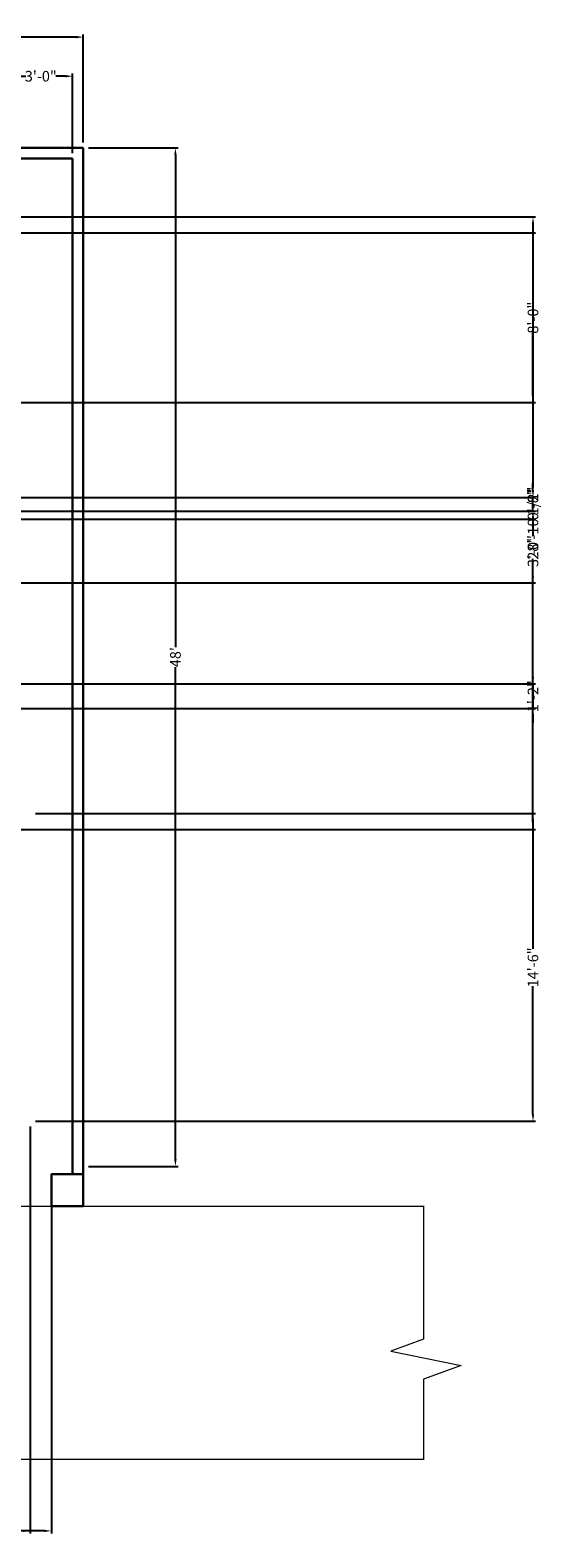
# Model space of a CAD drawing. Units: inches. Extents: x 6704 to 7574, y 11759 to 12617.
# Tile 8 of 8: x 7281 to 7574, y 11764 to 12617. Entities that reach past the tile are written whole.
import ezdxf

# ---------------------------------------------------------------- set-up
doc = ezdxf.new("R2010")
doc.units = ezdxf.units.IN
doc.header["$MEASUREMENT"] = 0
for name, color, linetype, lineweight in [('A-ANNO-SYMB', 8, 'Continuous', 18), ('C-PROP', 7, 'Continuous', 30), ('C-ROAD', 8, 'Continuous', 20), ('YQ_DIM', 3, 'Continuous', 18)]:
    doc.layers.add(name, color=color, linetype=linetype, lineweight=lineweight)
doc.styles.get("Standard").update_dxf_attribs({"font": 'arial.ttf'})
doc.dimstyles.new('yqi0', dxfattribs={"dimscale": 0, "dimtxt": 6, "dimasz": 4, "dimexe": 1.5, "dimexo": 3, "dimgap": 0.5, "dimtad": 0, "dimdsep": 46, "dimlunit": 4, "dimtxsty": 'Standard', "dimcen": 0, "dimclrd": 256, "dimclre": 256, "dimclrt": 7, "dimadec": 1, "dimazin": 2, "dimtfac": 1, "dimtix": 1, "dimtmove": 2, "dimatfit": 2, "dimfxl": 1, "dimtolj": 1, "dimtzin": 0, "dimarcsym": 0})

# ---------------------------------------------------------------- blocks, each defined once
blk = doc.blocks.new('*D2')
at = {"layer": 'Defpoints', "color": 0, "transparency": 16777216}
for p in [(7311.07, 12612.93), (6879.07, 12550.26), (7311.07, 12550.26)]:
    blk.add_point(p, dxfattribs=at)
at = {"layer": 'YQ_DIM', "color": 0, "lineweight": -2, "transparency": 16777216}
for p, q in [((6879.07, 12553.26), (6879.07, 12614.43)), ((6883.07, 12612.93), (7089.48, 12612.93)), ((7307.07, 12612.93), (7100.66, 12612.93)), ((7311.07, 12553.26), (7311.07, 12614.43))]:
    blk.add_line(p, q, dxfattribs=at)
at = {"layer": 'YQ_DIM', "color": 0, "transparency": 16777216}
for points in [[(6883.07, 12613.6), (6883.07, 12612.27), (6879.07, 12612.93)], [(7307.07, 12613.6), (7307.07, 12612.27), (7311.07, 12612.93)]]:
    blk.add_solid(points, dxfattribs=at)
at = {"layer": 'YQ_DIM', "color": 0, "transparency": 16777216, "insert": (7095.07, 12612.93), "char_height": 6, "attachment_point": 5}
blk.add_mtext("\\A1;36'", dxfattribs=at)
blk = doc.blocks.new('*D3')
at = {"layer": 'Defpoints', "color": 0, "transparency": 16777216}
for p in [(7311.07, 12550.26), (7311.07, 11974.26), (7363.16, 11974.26)]:
    blk.add_point(p, dxfattribs=at)
at = {"layer": 'YQ_DIM', "color": 0, "lineweight": -2, "transparency": 16777216}
for p, q in [((7314.07, 12550.26), (7364.66, 12550.26)), ((7363.16, 12546.26), (7363.16, 12267.97)), ((7363.16, 11978.26), (7363.16, 12256.55)), ((7314.07, 11974.26), (7364.66, 11974.26))]:
    blk.add_line(p, q, dxfattribs=at)
at = {"layer": 'YQ_DIM', "color": 0, "transparency": 16777216}
for points in [[(7362.49, 12546.26), (7363.83, 12546.26), (7363.16, 12550.26)], [(7362.49, 11978.26), (7363.83, 11978.26), (7363.16, 11974.26)]]:
    blk.add_solid(points, dxfattribs=at)
at = {"layer": 'YQ_DIM', "color": 0, "transparency": 16777216, "insert": (7363.16, 12262.26), "char_height": 6, "attachment_point": 5, "rotation": 90}
blk.add_mtext("\\A1;48'", dxfattribs=at)
blk = doc.blocks.new('GATE-PIER-18')
blk.add_lwpolyline([(18, 0), (0, 0), (0, 18), (18, 18), (18, 6)], close=True)
blk = doc.blocks.new('ROAD-BREAK')
blk.add_lwpolyline([(18.36, 29.8), (18.36, 24.82), (0, 18.15), (39.74, 9.9), (18.36, 2.15), (18.36, 0)])
blk = doc.blocks.new('*D58')
at = {"layer": 'Defpoints', "color": 0, "transparency": 16777216}
for p in [(7305.07, 12590.81), (7305.07, 12544.26), (7269.07, 12511.26)]:
    blk.add_point(p, dxfattribs=at)
at = {"layer": 'YQ_DIM', "lineweight": -2, "transparency": 16777216}
for p, q in [((7269.07, 12514.26), (7269.07, 12592.31)), ((7273.07, 12590.81), (7278.6, 12590.81)), ((7301.07, 12590.81), (7295.55, 12590.81)), ((7305.07, 12547.26), (7305.07, 12592.31))]:
    blk.add_line(p, q, dxfattribs=at)
at = {"layer": 'YQ_DIM', "transparency": 16777216}
for points in [[(7273.07, 12591.47), (7273.07, 12590.14), (7269.07, 12590.81)], [(7301.07, 12591.47), (7301.07, 12590.14), (7305.07, 12590.81)]]:
    blk.add_solid(points, dxfattribs=at)
at = {"layer": 'YQ_DIM', "color": 7, "transparency": 16777216, "insert": (7287.07, 12590.81), "char_height": 6, "attachment_point": 5}
blk.add_mtext('\\A1;3\'-0"', dxfattribs=at)
blk = doc.blocks.new('*D61')
at = {"layer": 'Defpoints', "color": 0, "transparency": 16777216}
for p in [(7117.57, 12502.26), (7565.25, 12502.26), (7117.57, 12406.26)]:
    blk.add_point(p, dxfattribs=at)
at = {"layer": 'YQ_DIM', "lineweight": -2, "transparency": 16777216}
for p, q in [((7120.57, 12502.26), (7566.75, 12502.26)), ((7565.25, 12498.26), (7565.25, 12462.74)), ((7565.25, 12410.26), (7565.25, 12445.78)), ((7120.57, 12406.26), (7566.75, 12406.26))]:
    blk.add_line(p, q, dxfattribs=at)
at = {"layer": 'YQ_DIM', "transparency": 16777216}
for points in [[(7564.58, 12498.26), (7565.91, 12498.26), (7565.25, 12502.26)], [(7564.58, 12410.26), (7565.91, 12410.26), (7565.25, 12406.26)]]:
    blk.add_solid(points, dxfattribs=at)
at = {"layer": 'YQ_DIM', "color": 7, "transparency": 16777216, "insert": (7565.25, 12454.26), "char_height": 6, "attachment_point": 5, "rotation": 90}
blk.add_mtext('\\A1;8\'-0"', dxfattribs=at)
blk = doc.blocks.new('*D63')
at = {"layer": 'Defpoints', "color": 0, "transparency": 16777216}
for p in [(7269.07, 12511.26), (7565.25, 12511.26), (7269.07, 12164.76)]:
    blk.add_point(p, dxfattribs=at)
at = {"layer": 'YQ_DIM', "lineweight": -2, "transparency": 16777216}
for p, q in [((7272.07, 12511.26), (7566.75, 12511.26)), ((7565.25, 12507.26), (7565.25, 12358.19)), ((7565.25, 12168.76), (7565.25, 12317.83)), ((7272.07, 12164.76), (7566.75, 12164.76))]:
    blk.add_line(p, q, dxfattribs=at)
at = {"layer": 'YQ_DIM', "transparency": 16777216}
for points in [[(7564.58, 12507.26), (7565.91, 12507.26), (7565.25, 12511.26)], [(7564.58, 12168.76), (7565.91, 12168.76), (7565.25, 12164.76)]]:
    blk.add_solid(points, dxfattribs=at)
at = {"layer": 'YQ_DIM', "color": 7, "transparency": 16777216, "insert": (7565.25, 12338.01), "char_height": 6, "attachment_point": 5, "rotation": 90}
blk.add_mtext('\\A1;28\'-10 1/2"', dxfattribs=at)
blk = doc.blocks.new('*D68')
at = {"layer": 'Defpoints', "color": 0, "transparency": 16777216}
for p in [(6927.07, 12340.26), (7565.25, 12340.26), (6927.07, 12304.26)]:
    blk.add_point(p, dxfattribs=at)
at = {"layer": 'YQ_DIM', "lineweight": -2, "transparency": 16777216}
for p, q in [((6930.07, 12340.26), (7566.75, 12340.26)), ((7565.25, 12336.26), (7565.25, 12330.73)), ((7565.25, 12308.26), (7565.25, 12313.78)), ((6930.07, 12304.26), (7566.75, 12304.26))]:
    blk.add_line(p, q, dxfattribs=at)
at = {"layer": 'YQ_DIM', "transparency": 16777216}
for points in [[(7564.58, 12336.26), (7565.91, 12336.26), (7565.25, 12340.26)], [(7564.58, 12308.26), (7565.91, 12308.26), (7565.25, 12304.26)]]:
    blk.add_solid(points, dxfattribs=at)
at = {"layer": 'YQ_DIM', "color": 7, "transparency": 16777216, "insert": (7565.25, 12322.26), "char_height": 6, "attachment_point": 5, "rotation": 90}
blk.add_mtext('\\A1;3\'-0"', dxfattribs=at)
blk = doc.blocks.new('*D69')
at = {"layer": 'Defpoints', "color": 0, "transparency": 16777216}
for p in [(7122.57, 12247.15), (7122.57, 12233.15), (7565.25, 12233.15)]:
    blk.add_point(p, dxfattribs=at)
at = {"layer": 'YQ_DIM', "lineweight": -2, "transparency": 16777216}
for p, q in [((7565.25, 12251.15), (7565.25, 12255.15)), ((7125.57, 12247.15), (7566.75, 12247.15)), ((7565.25, 12247.15), (7565.25, 12233.15)), ((7125.57, 12233.15), (7566.75, 12233.15)), ((7565.25, 12229.15), (7565.25, 12225.15))]:
    blk.add_line(p, q, dxfattribs=at)
at = {"layer": 'YQ_DIM', "transparency": 16777216}
for points in [[(7564.58, 12251.15), (7565.91, 12251.15), (7565.25, 12247.15)], [(7564.58, 12229.15), (7565.91, 12229.15), (7565.25, 12233.15)]]:
    blk.add_solid(points, dxfattribs=at)
at = {"layer": 'YQ_DIM', "color": 7, "transparency": 16777216, "insert": (7565.25, 12240.15), "char_height": 6, "attachment_point": 5, "rotation": 90}
blk.add_mtext('\\A1;1\'-2"', dxfattribs=at)
blk = doc.blocks.new('*D70')
at = {"layer": 'Defpoints', "color": 0, "transparency": 16777216}
for p in [(7122.07, 11969.76), (7293.07, 11969.76), (7293.07, 11768.08)]:
    blk.add_point(p, dxfattribs=at)
at = {"layer": 'YQ_DIM', "lineweight": -2, "transparency": 16777216}
for p, q in [((7122.07, 11966.76), (7122.07, 11766.58)), ((7293.07, 11966.76), (7293.07, 11766.58)), ((7126.07, 11768.08), (7197.05, 11768.08)), ((7289.07, 11768.08), (7218.1, 11768.08))]:
    blk.add_line(p, q, dxfattribs=at)
at = {"layer": 'YQ_DIM', "transparency": 16777216}
for points in [[(7126.07, 11768.74), (7126.07, 11767.41), (7122.07, 11768.08)], [(7289.07, 11768.74), (7289.07, 11767.41), (7293.07, 11768.08)]]:
    blk.add_solid(points, dxfattribs=at)
at = {"layer": 'YQ_DIM', "color": 7, "transparency": 16777216, "insert": (7207.57, 11768.08), "char_height": 6, "attachment_point": 5}
blk.add_mtext('\\A1;14\'-3"', dxfattribs=at)
blk = doc.blocks.new('*D72')
at = {"layer": 'Defpoints', "color": 0, "transparency": 16777216}
for p in [(7113.07, 11999.76), (7281.07, 11999.76), (7281.07, 11768.08)]:
    blk.add_point(p, dxfattribs=at)
at = {"layer": 'YQ_DIM', "lineweight": -2, "transparency": 16777216}
for p, q in [((7113.07, 11996.76), (7113.07, 11766.58)), ((7281.07, 11996.76), (7281.07, 11766.58)), ((7117.07, 11768.08), (7186.55, 11768.08)), ((7277.07, 11768.08), (7207.6, 11768.08))]:
    blk.add_line(p, q, dxfattribs=at)
at = {"layer": 'YQ_DIM', "transparency": 16777216}
for points in [[(7117.07, 11768.74), (7117.07, 11767.41), (7113.07, 11768.08)], [(7277.07, 11768.74), (7277.07, 11767.41), (7281.07, 11768.08)]]:
    blk.add_solid(points, dxfattribs=at)
at = {"layer": 'YQ_DIM', "color": 7, "transparency": 16777216, "insert": (7197.07, 11768.08), "char_height": 6, "attachment_point": 5}
blk.add_mtext('\\A1;14\'-0"', dxfattribs=at)
blk = doc.blocks.new('*D73')
at = {"layer": 'Defpoints', "color": 0, "transparency": 16777216}
for p in [(7281.07, 12173.76), (7565.25, 12173.76), (7281.07, 11999.76)]:
    blk.add_point(p, dxfattribs=at)
at = {"layer": 'YQ_DIM', "lineweight": -2, "transparency": 16777216}
for p, q in [((7284.07, 12173.76), (7566.75, 12173.76)), ((7565.25, 12169.76), (7565.25, 12097.28)), ((7565.25, 12003.76), (7565.25, 12076.23)), ((7284.07, 11999.76), (7566.75, 11999.76))]:
    blk.add_line(p, q, dxfattribs=at)
at = {"layer": 'YQ_DIM', "transparency": 16777216}
for points in [[(7564.58, 12169.76), (7565.91, 12169.76), (7565.25, 12173.76)], [(7564.58, 12003.76), (7565.91, 12003.76), (7565.25, 11999.76)]]:
    blk.add_solid(points, dxfattribs=at)
at = {"layer": 'YQ_DIM', "color": 7, "transparency": 16777216, "insert": (7565.25, 12086.76), "char_height": 6, "attachment_point": 5, "rotation": 90}
blk.add_mtext('\\A1;14\'-6"', dxfattribs=at)
blk = doc.blocks.new('*D82')
at = {"layer": 'Defpoints', "color": 0, "transparency": 16777216}
for p in [(7117.57, 12352.63), (7565.25, 12352.63), (7122.07, 12344.76)]:
    blk.add_point(p, dxfattribs=at)
at = {"layer": 'YQ_DIM', "lineweight": -2, "transparency": 16777216}
for p, q in [((7565.25, 12356.63), (7565.25, 12360.63)), ((7120.57, 12352.63), (7566.75, 12352.63)), ((7565.25, 12344.76), (7565.25, 12352.63)), ((7125.07, 12344.76), (7566.75, 12344.76)), ((7565.25, 12340.76), (7565.25, 12336.76))]:
    blk.add_line(p, q, dxfattribs=at)
at = {"layer": 'YQ_DIM', "transparency": 16777216}
for points in [[(7564.58, 12356.63), (7565.91, 12356.63), (7565.25, 12352.63)], [(7564.58, 12340.76), (7565.91, 12340.76), (7565.25, 12344.76)]]:
    blk.add_solid(points, dxfattribs=at)
at = {"layer": 'YQ_DIM', "color": 7, "transparency": 16777216, "insert": (7565.25, 12348.69), "char_height": 6, "attachment_point": 5, "rotation": 90}
blk.add_mtext('\\A1;0\'-8"', dxfattribs=at)

msp = doc.modelspace()

# ---------------------------------------------------------------- linework, layer by layer
at = {"layer": 'C-PROP'}
for p, q in [((6879.073, 12550.257), (7311.073, 12550.257)), ((6885.073, 12544.257), (7305.073, 12544.257)), ((7305.073, 11969.757), (7305.073, 12544.257)), ((7311.073, 11951.757), (7311.073, 12550.257)), ((7305.073, 11951.757), (7311.073, 11951.757))]:
    msp.add_line(p, q, dxfattribs=at)
at = {"layer": 'C-ROAD'}
for p, q in [((6771.883, 11951.757), (7503.792, 11951.757)), ((7503.323, 11951.757), (7503.323, 11876.472)), ((7503.323, 11853.793), (7503.323, 11808.627)), ((6771.883, 11808.627), (7503.792, 11808.627))]:
    msp.add_line(p, q, dxfattribs=at)

# ---------------------------------------------------------------- block references
at = {"layer": 'A-ANNO-SYMB'}
msp.add_blockref('ROAD-BREAK', (7484.96, 11851.647), dxfattribs=at)
at = {"layer": 'C-PROP'}
msp.add_blockref('GATE-PIER-18', (7293.073, 11951.757), dxfattribs=at)

# ---------------------------------------------------------------- dimensions: what is measured, and where the dimension line sits
at = {"layer": 'YQ_DIM'}
for p1, p2, distance, picture, middle in [((6879.073, 12550.257), (7311.073, 12550.257), 62.676, '*D2', (7095.073, 12612.934)), ((7311.073, 12550.257), (7311.073, 11974.257), 52.089, '*D3', (7363.162, 12262.257))]:
    dim = msp.add_aligned_dim(p1=p1, p2=p2, distance=distance, dimstyle='yqi0', override={"dimscale": 1, "dimclrd": 0, "dimclre": 0, "dimclrt": 0}, dxfattribs=at)
    dim.commit()
    dim.dimension.update_dxf_attribs({"geometry": picture, "text_midpoint": middle})
for base, p1, p2, picture, middle in [((7305.073, 12590.807), (7269.073, 12511.257), (7305.073, 12544.257), '*D58', (7287.073, 12590.807)), ((7281.073, 11768.077), (7113.073, 11999.757), (7281.073, 11999.757), '*D72', (7197.073, 11768.077)), ((7293.073, 11768.077), (7122.073, 11969.757), (7293.073, 11969.757), '*D70', (7207.573, 11768.077))]:
    dim = msp.add_linear_dim(base=base, p1=p1, p2=p2, dimstyle='yqi0', override={"dimscale": 1, "dimdec": 1, "dimzin": 1, "dimfrac": 2}, dxfattribs=at)
    dim.commit()
    dim.dimension.update_dxf_attribs({"geometry": picture, "text_midpoint": middle})
for base, p1, p2, picture, middle in [((7565.248, 12511.257), (7269.073, 12164.757), (7269.073, 12511.257), '*D63', (7565.248, 12338.007)), ((7565.248, 12502.257), (7117.573, 12406.257), (7117.573, 12502.257), '*D61', (7565.248, 12454.257)), ((7565.248, 12352.631), (7122.073, 12344.757), (7117.573, 12352.631), '*D82', (7565.248, 12348.694)), ((7565.248, 12340.257), (6927.073, 12304.257), (6927.073, 12340.257), '*D68', (7565.248, 12322.257)), ((7565.248, 12233.154), (7122.573, 12247.154), (7122.573, 12233.154), '*D69', (7565.248, 12240.154)), ((7565.248, 12173.757), (7281.073, 11999.757), (7281.073, 12173.757), '*D73', (7565.248, 12086.757))]:
    dim = msp.add_linear_dim(base=base, p1=p1, p2=p2, angle=90, dimstyle='yqi0', override={"dimscale": 1, "dimdec": 1, "dimzin": 1, "dimfrac": 2}, dxfattribs=at)
    dim.commit()
    dim.dimension.update_dxf_attribs({"geometry": picture, "text_midpoint": middle})

doc.saveas('drawing.dxf')
